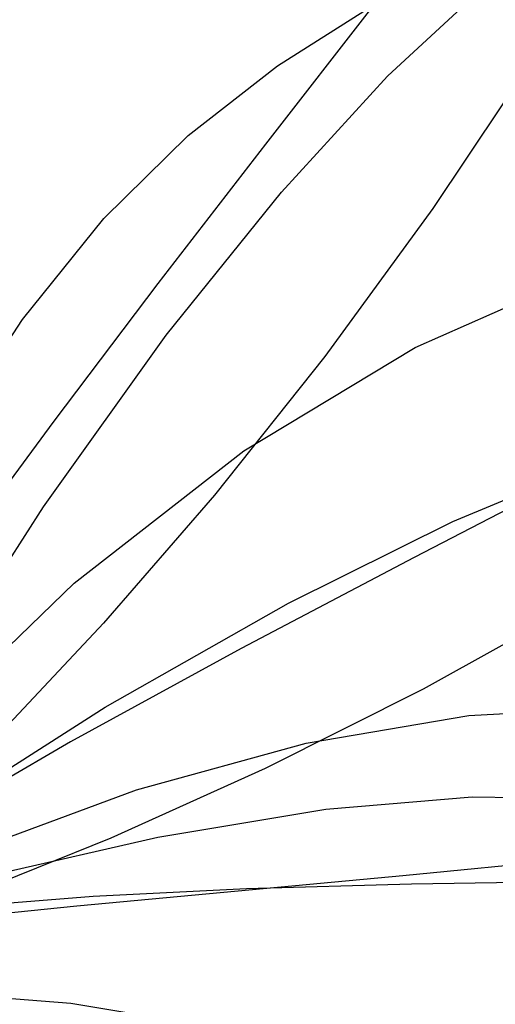
# Model space of a CAD drawing. Units: inches. Extents: x 3590 to 5167, y 65 to 1917.
# Tile 93 of 100: x 5053.48 to 5058.39, y 1778.86 to 1789.03. Entities that reach past the tile are written whole.
import ezdxf

# ---------------------------------------------------------------- set-up
doc = ezdxf.new("R2010")
doc.units = ezdxf.units.IN
for name, color, linetype, lineweight in [('A-ANNO-DIMS', 2, 'Continuous', 18), ('A-FLOR-PATT', 8, 'Continuous', 13), ('L-PLNT', 94, 'Continuous', 18)]:
    doc.layers.add(name, color=color, linetype=linetype, lineweight=lineweight)
doc.layers.add('DIENHOA', color=3, linetype='Continuous')
doc.styles.get("Standard").update_dxf_attribs({"font": 'arial.ttf'})
doc.dimstyles.new('ISO-25', dxfattribs={"dimtxt": 9, "dimasz": 2.5, "dimexe": 1.25, "dimexo": 0.625, "dimtad": 1, "dimdec": 1, "dimlunit": 3, "dimtxsty": 'Standard', "dimcen": 2.5, "dimadec": 0, "dimazin": 0, "dimtfac": 1, "dimtdec": 1, "dimtmove": 0, "dimatfit": 3, "dimfxl": 1, "dimarcsym": 0})

# ---------------------------------------------------------------- blocks, each defined once
blk = doc.blocks.new('Cay03_mb')
at = {"layer": 'DIENHOA'}
for p, q in [((290.63, 243.24), (363.38, 275.41)), ((218.51, 199.79), (290.63, 243.24)), ((146.96, 144.09), (218.51, 199.79)), ((363.69, 192.89), (290.19, 154.87)), ((290.19, 154.87), (217.38, 116.61)), ((75.94, 75.22), (146.96, 144.09)), ((217.38, 116.61), (145.48, 77.28)), ((145.48, 77.28), (74.74, 36.09)), ((252.97, 48.94), (314.63, 54.14)), ((314.63, 54.14), (369.18, 53.28)), ((182.2, 37.2), (252.97, 48.94)), ((100.34, 18.45), (182.2, 37.2)), ((289.03, 17.44), (219.62, 15.45)), ((361.61, 18.5), (289.03, 17.44)), ((219.62, 15.45), (154.97, 12.22)), ((154.97, 12.22), (96.66, 7.47))]:
    blk.add_line(p, q, dxfattribs=at)
for points in [[(384.28, 437.45), (342.25, 367.83), (298.14, 301.71), (252.56, 239.37), (206.11, 181.11), (159.39, 127.21), (113.01, 77.96), (67.57, 33.64), (23.69, -5.44)], [(23.69, -5.44), (79.88, 91.71), (134.12, 176.21), (185.81, 248.4), (234.31, 308.65), (279.02, 357.33), (319.33, 394.78), (354.62, 421.37), (384.28, 437.45)], [(273.24, 387.35), (227.6, 328.83), (182.25, 270.12), (138.39, 212.28), (97.23, 156.36), (59.96, 103.43), (27.8, 54.57), (1.94, 10.82), (-16.39, -26.73)], [(-16.39, -26.73), (21.41, 64.22), (57.05, 140.27), (91.37, 203.26), (125.24, 255.05), (159.51, 297.5), (195.03, 332.46), (232.65, 361.79), (273.24, 387.35)], [(496.74, 224.01), (429.38, 178.44), (361.6, 136.93), (294.07, 99.46), (227.46, 66.07), (162.44, 36.74), (99.68, 11.49), (39.84, -9.67), (-16.39, -26.73)], [(-16.39, -26.73), (75.38, 37.88), (160.06, 91.82), (237.27, 135.67), (306.57, 170.01), (367.58, 195.44), (419.88, 212.52), (463.07, 221.85), (496.74, 224.01)], [(23.69, -5.44), (99.27, 29.67), (173.22, 57.09), (244.79, 76.69), (313.26, 88.31), (377.88, 91.81), (437.93, 87.02), (492.67, 73.8), (541.37, 52)], [(541.37, 52), (484.11, 42.89), (421.18, 34.83), (354.36, 27.58), (285.41, 20.89), (216.1, 14.49), (148.2, 8.14), (83.47, 1.58), (23.69, -5.44)], [(-16.39, -26.73), (66.95, -26.58), (145.58, -32.71), (218.77, -44.94), (285.79, -63.12), (345.92, -87.06), (398.42, -116.6), (442.57, -151.57), (477.63, -191.79)]]:
    blk.add_lwpolyline(points, dxfattribs=at)
blk = doc.blocks.new('*D322')
at = {"layer": 'A-ANNO-DIMS', "color": 0, "lineweight": -2, "transparency": 16777216}
for p, q in [((5035.744, 1766.184), (5035.744, 1761.199)), ((5064.812, 1766.184), (5064.812, 1761.199)), ((5038.244, 1762.449), (5062.312, 1762.449)), ((5064.812, 1762.449), (5166.991, 1762.449))]:
    blk.add_line(p, q, dxfattribs=at)
at = {"layer": 'A-ANNO-DIMS', "color": 0, "transparency": 16777216}
for points in [[(5038.244, 1762.866), (5038.244, 1762.032), (5035.744, 1762.449)], [(5062.312, 1762.866), (5062.312, 1762.032), (5064.812, 1762.449)]]:
    blk.add_solid(points, dxfattribs=at)
at = {"layer": 'Defpoints', "color": 0, "transparency": 16777216}
for p in [(5035.744, 1766.809), (5064.812, 1766.809), (5064.812, 1762.449)]:
    blk.add_point(p, dxfattribs=at)
at = {"layer": 'A-ANNO-DIMS', "color": 0, "transparency": 16777216, "insert": (5117.152, 1767.669), "char_height": 9, "attachment_point": 5}
blk.add_mtext('PLANT 2\'-5" TYP.', dxfattribs=at)
blk = doc.blocks.new('*D323')
at = {"layer": 'A-ANNO-DIMS', "color": 0, "lineweight": -2, "transparency": 16777216}
for p, q in [((5069.172, 1795.216), (5069.172, 1874.95)), ((5065.437, 1795.216), (5070.422, 1795.216)), ((5069.172, 1769.309), (5069.172, 1792.716)), ((5065.437, 1766.809), (5070.422, 1766.809))]:
    blk.add_line(p, q, dxfattribs=at)
at = {"layer": 'A-ANNO-DIMS', "color": 0, "transparency": 16777216}
for points in [[(5068.756, 1792.716), (5069.589, 1792.716), (5069.172, 1795.216)], [(5068.756, 1769.309), (5069.589, 1769.309), (5069.172, 1766.809)]]:
    blk.add_solid(points, dxfattribs=at)
at = {"layer": 'Defpoints', "color": 0, "transparency": 16777216}
for p in [(5064.812, 1795.216), (5069.172, 1795.216), (5064.812, 1766.809)]:
    blk.add_point(p, dxfattribs=at)
at = {"layer": 'A-ANNO-DIMS', "color": 0, "transparency": 16777216, "insert": (5063.894, 1836.333), "char_height": 9, "attachment_point": 5, "rotation": 90}
blk.add_mtext('2\'-4 1/2" TYP.', dxfattribs=at)

msp = doc.modelspace()

# ---------------------------------------------------------------- hatches: boundary and pattern name
at = {"layer": 'A-FLOR-PATT', "transparency": 33554687}
h = msp.add_hatch(dxfattribs=at)
h.set_pattern_fill('AR-HBONE', color=256, scale=0.2)
h.set_pattern_definition([(45, (-588.972, 0), (0, 28.73682), [60.96, -20.32]), (135, (-574.604, 14.368), (3e-15, 28.73682), [60.96, -20.32])])
h.paths.add_polyline_path([(5071.274, 1796.999), (4933.274, 1796.999), (4933.274, 1753.999), (4962.774, 1753.999, -0.414214), (4928.774, 1719.999), (4933.274, 1718.999), (4933.274, 1334.999), (5071.274, 1334.999)])
h.paths.add_polyline_path([(4951.78, 1521.077), (4951.715, 1521.04), (4951.563, 1520.895)], flags=16)
h.paths.add_polyline_path([(4952.267, 1521.376), (4952.198, 1521.371), (4952.198, 1521.356)], flags=0)
h.paths.add_polyline_path([(4967.051, 1529.728), (4965.231, 1528.694), (4963.411, 1527.714), (4961.756, 1526.851), (4963.589, 1527.449), (4964.036, 1527.478), (4962.975, 1527.249), (4961.76, 1526.852), (4959.792, 1525.834), (4958.005, 1524.895), (4956.24, 1523.93), (4954.504, 1522.919), (4954.129, 1522.682), (4953.361, 1521.997), (4953.366, 1521.998), (4953.605, 1522.064), (4955.106, 1522.761), (4956.921, 1523.434), (4958.678, 1523.915), (4960.358, 1524.2), (4961.945, 1524.286), (4964.171, 1524.108), (4965.958, 1523.309), (4963.863, 1522.976), (4965.187, 1522.499), (4963.366, 1522.497), (4961.545, 1522.487), (4959.764, 1522.461), (4958.304, 1522.419), (4957.974, 1522.388), (4956.307, 1522.232), (4954.718, 1522.071), (4953.251, 1521.899), (4953.525, 1521.623), (4954.331, 1521.379), (4956.243, 1521.23), (4958.039, 1520.93), (4959.684, 1520.483), (4961.16, 1519.896), (4963.107, 1518.8), (4964.393, 1517.325), (4962.973, 1517.726), (4964.558, 1516.661), (4965.407, 1515.708), (4963.507, 1516.322), (4961.68, 1517.005), (4959.935, 1517.745), (4958.282, 1518.528), (4956.732, 1519.343), (4955.295, 1520.175), (4954.672, 1520.572), (4954.513, 1520.627), (4955.658, 1519.318), (4956.703, 1517.982), (4957.644, 1516.647), (4958.485, 1515.334), (4959.55, 1513.524), (4960.438, 1511.769), (4958.841, 1513.62), (4957.452, 1515.325), (4955.819, 1517.459), (4956.665, 1515.448), (4957.111, 1513.923), (4957.447, 1511.714), (4957.076, 1509.793), (4956.538, 1511.11), (4955.992, 1512.569), (4955.444, 1514.125), (4954.898, 1515.735), (4954.357, 1517.356), (4953.824, 1518.943), (4953.305, 1520.452), (4953.065, 1521.116), (4952.971, 1521.146), (4952.949, 1521.086), (4952.73, 1520.199), (4953.37, 1518.024), (4953.757, 1516.373), (4954.051, 1514.765), (4954.264, 1513.221), (4954.471, 1511.131), (4954.497, 1510.402), (4954.409, 1511.76), (4954.264, 1513.221), (4954.051, 1514.765), (4953.757, 1516.373), (4953.37, 1518.024), (4952.877, 1519.698), (4952.716, 1520.141), (4952.533, 1519.059), (4952.374, 1517.789), (4952.219, 1516.312), (4952.046, 1514.6), (4951.833, 1512.626), (4951.557, 1510.363), (4951.203, 1512.168), (4950.852, 1514.339), (4950.985, 1516.376), (4951.66, 1518.286), (4952.593, 1520.481), (4952.357, 1521.13), (4951.855, 1520.328), (4950.839, 1518.908), (4949.777, 1517.587), (4948.916, 1516.617), (4948.111, 1515.256), (4947.089, 1513.554), (4945.889, 1511.615), (4946.326, 1513.402), (4946.562, 1514.249), (4945.528, 1513.327), (4944.581, 1512.531), (4946.018, 1514.508), (4947.204, 1516.048), (4947.893, 1517.313), (4949.307, 1518.764), (4950.414, 1519.767), (4950.451, 1519.806), (4952.267, 1521.376), (4951.645, 1521.493), (4950.404, 1521.18), (4948.044, 1520.359), (4946.119, 1519.452), (4944.572, 1518.475), (4943.35, 1517.443), (4941.997, 1515.92), (4941.661, 1515.275), (4942.813, 1516.99), (4944.572, 1518.475), (4946.119, 1519.452), (4948.044, 1520.359), (4950.404, 1521.18), (4951.645, 1521.493), (4949.647, 1521.868), (4948.6, 1521.756), (4947.126, 1521.57), (4945.42, 1521.348), (4943.45, 1521.105), (4941.183, 1520.856), (4942.86, 1521.613), (4943.873, 1522.03), (4942.952, 1521.909), (4941.41, 1521.485), (4939.543, 1520.67), (4938.968, 1520.226), (4940.733, 1521.299), (4942.952, 1521.909), (4943.702, 1522.008), (4945.894, 1522.7), (4947.565, 1522.714), (4948.921, 1522.566), (4951.131, 1522.183), (4950.971, 1522.297), (4948.129, 1523.006), (4946.035, 1523.707), (4944.232, 1524.521), (4942.707, 1525.461), (4941.444, 1526.537), (4940.43, 1527.761), (4939.649, 1529.143), (4941.421, 1528.122), (4943.147, 1527.132), (4944.841, 1526.175), (4946.514, 1525.25), (4948.179, 1524.359), (4948.365, 1524.263), (4946.475, 1526.045), (4945.181, 1527.54), (4944.19, 1529.033), (4943.496, 1530.54), (4943.278, 1531.36), (4942.498, 1531.919), (4943.114, 1531.762), (4942.959, 1533.659), (4944.14, 1531.989), (4944.612, 1531.323), (4946.202, 1530.463), (4947.486, 1529.509), (4948.79, 1528.226), (4950.368, 1526.237), (4949.485, 1528.155), (4948.851, 1530.123), (4948.491, 1532.041), (4948.381, 1533.918), (4948.501, 1535.76), (4948.827, 1537.573), (4949.418, 1535.565), (4949.957, 1533.569), (4950.464, 1531.586), (4950.961, 1529.617), (4951.391, 1527.954), (4951.724, 1530.687), (4952.201, 1532.58), (4952.889, 1534.33), (4953.77, 1535.951), (4954.827, 1537.46), (4954.521, 1535.39), (4954.273, 1533.937), (4955.58, 1535.663), (4956.748, 1536.739), (4956.159, 1534.78), (4955.589, 1532.873), (4955.043, 1531.006), (4954.525, 1529.166), (4954.038, 1527.341), (4953.638, 1525.733), (4953.611, 1525.586), (4953.398, 1524.166), (4953.382, 1524.009), (4954.07, 1525.476), (4954.912, 1527.022), (4956.136, 1528.894), (4957.847, 1530.577), (4959.376, 1531.54), (4958.256, 1530.104), (4957.143, 1528.663), (4956.066, 1527.243), (4955.056, 1525.871), (4954.141, 1524.571), (4953.352, 1523.372), (4953.311, 1523.303), (4953.273, 1522.925), (4953.261, 1522.382), (4954.103, 1523.373), (4954.63, 1524.284), (4955.961, 1526.358), (4957.23, 1528.13), (4958.421, 1529.609), (4960.037, 1531.368), (4961.374, 1532.375), (4962.101, 1532.77), (4961.07, 1531.061), (4959.987, 1529.438), (4958.869, 1527.908), (4958.15, 1527.007), (4959.803, 1528.003), (4961.589, 1528.793), (4963.391, 1529.328), (4965.211, 1529.632)], flags=16)
h.paths.add_polyline_path([(4962.944, 1523.182), (4961.107, 1523.422), (4960.392, 1523.362), (4962.35, 1523.331)], flags=0)
h.paths.add_polyline_path([(5049.541, 1584.551), (5049.476, 1584.515), (5049.325, 1584.37)], flags=16)
h.paths.add_polyline_path([(5050.028, 1584.851), (5049.959, 1584.845), (5049.959, 1584.83)], flags=0)
h.paths.add_polyline_path([(5042.333, 1581.949), (5043.88, 1582.926), (5045.806, 1583.833), (5048.165, 1584.654), (5049.406, 1584.967), (5047.408, 1585.342), (5046.361, 1585.231), (5044.888, 1585.044), (5043.181, 1584.822), (5041.211, 1584.579), (5038.944, 1584.33), (5040.622, 1585.087), (5041.634, 1585.504), (5040.713, 1585.383), (5039.171, 1584.959), (5037.304, 1584.144), (5036.729, 1583.7), (5038.494, 1584.773), (5040.713, 1585.383), (5041.463, 1585.482), (5043.655, 1586.174), (5045.326, 1586.188), (5046.682, 1586.04), (5048.893, 1585.657), (5048.732, 1585.771), (5045.891, 1586.48), (5043.796, 1587.181), (5041.994, 1587.996), (5040.468, 1588.935), (5039.205, 1590.011), (5038.191, 1591.235), (5037.41, 1592.617), (5039.182, 1591.596), (5040.909, 1590.607), (5042.602, 1589.649), (5044.275, 1588.724), (5045.94, 1587.833), (5046.126, 1587.738), (5044.237, 1589.519), (5042.942, 1591.015), (5041.952, 1592.508), (5041.257, 1594.014), (5041.039, 1594.834), (5040.26, 1595.393), (5040.875, 1595.237), (5040.721, 1597.133), (5041.901, 1595.463), (5042.373, 1594.798), (5043.963, 1593.938), (5045.247, 1592.983), (5046.552, 1591.701), (5048.129, 1589.712), (5047.247, 1591.63), (5046.613, 1593.597), (5046.252, 1595.515), (5046.142, 1597.392), (5046.262, 1599.234), (5046.588, 1601.047), (5047.179, 1599.039), (5047.718, 1597.043), (5048.225, 1595.06), (5048.722, 1593.091), (5049.152, 1591.429), (5049.485, 1594.161), (5049.962, 1596.054), (5050.65, 1597.804), (5051.532, 1599.425), (5052.589, 1600.934), (5052.283, 1598.864), (5052.034, 1597.411), (5053.341, 1599.137), (5054.509, 1600.213), (5053.92, 1598.254), (5053.35, 1596.348), (5052.805, 1594.48), (5052.286, 1592.64), (5051.799, 1590.815), (5051.4, 1589.207), (5051.373, 1589.06), (5051.159, 1587.64), (5051.143, 1587.483), (5051.831, 1588.95), (5052.673, 1590.496), (5053.898, 1592.368), (5055.608, 1594.051), (5057.137, 1595.014), (5056.017, 1593.578), (5054.904, 1592.137), (5053.828, 1590.717), (5052.817, 1589.345), (5051.902, 1588.046), (5051.113, 1586.846), (5051.072, 1586.777), (5051.034, 1586.399), (5051.022, 1585.856), (5051.864, 1586.847), (5052.391, 1587.758), (5053.723, 1589.832), (5054.991, 1591.604), (5056.182, 1593.083), (5057.798, 1594.842), (5059.135, 1595.849), (5059.863, 1596.244), (5058.831, 1594.535), (5057.749, 1592.912), (5056.63, 1591.382), (5055.912, 1590.482), (5057.564, 1591.477), (5059.35, 1592.267), (5061.152, 1592.802), (5062.972, 1593.106), (5064.812, 1593.203), (5062.992, 1592.169), (5061.172, 1591.188), (5059.518, 1590.325), (5061.35, 1590.924), (5061.797, 1590.952), (5060.737, 1590.723), (5059.521, 1590.326), (5057.553, 1589.308), (5055.766, 1588.369), (5054.002, 1587.404), (5052.265, 1586.393), (5051.891, 1586.156), (5051.122, 1585.471), (5051.127, 1585.472), (5051.366, 1585.538), (5052.867, 1586.235), (5054.682, 1586.908), (5056.439, 1587.389), (5058.12, 1587.675), (5059.706, 1587.76), (5061.933, 1587.583), (5063.719, 1586.783), (5061.624, 1586.45), (5062.949, 1585.973), (5061.127, 1585.971), (5059.307, 1585.961), (5057.525, 1585.935), (5056.065, 1585.893), (5055.735, 1585.862), (5054.068, 1585.707), (5052.479, 1585.546), (5051.012, 1585.373), (5051.286, 1585.097), (5052.092, 1584.853), (5054.004, 1584.704), (5055.8, 1584.404), (5057.446, 1583.958), (5058.921, 1583.37), (5060.868, 1582.274), (5062.154, 1580.799), (5060.734, 1581.2), (5062.32, 1580.135), (5063.168, 1579.182), (5061.269, 1579.796), (5059.441, 1580.479), (5057.696, 1581.219), (5056.043, 1582.003), (5054.493, 1582.817), (5053.057, 1583.649), (5052.433, 1584.047), (5052.274, 1584.101), (5053.42, 1582.793), (5054.464, 1581.457), (5055.405, 1580.121), (5056.247, 1578.809), (5057.311, 1576.998), (5058.199, 1575.244), (5056.602, 1577.094), (5055.213, 1578.799), (5053.58, 1580.933), (5054.427, 1578.922), (5054.872, 1577.397), (5055.208, 1575.189), (5054.838, 1573.267), (5054.299, 1574.584), (5053.754, 1576.043), (5053.206, 1577.599), (5052.659, 1579.209), (5052.118, 1580.83), (5051.585, 1582.417), (5051.066, 1583.927), (5050.826, 1584.59), (5050.733, 1584.62), (5050.711, 1584.561), (5050.491, 1583.673), (5051.131, 1581.498), (5051.518, 1579.847), (5051.813, 1578.24), (5052.026, 1576.695), (5052.233, 1574.605), (5052.258, 1573.876), (5052.17, 1575.234), (5052.026, 1576.695), (5051.813, 1578.24), (5051.518, 1579.847), (5051.131, 1581.498), (5050.638, 1583.172), (5050.477, 1583.615), (5050.294, 1582.533), (5050.136, 1581.263), (5049.981, 1579.786), (5049.807, 1578.074), (5049.594, 1576.1), (5049.318, 1573.837), (5048.965, 1575.642), (5048.613, 1577.813), (5048.747, 1579.85), (5049.421, 1581.76), (5050.354, 1583.955), (5050.118, 1584.604), (5049.616, 1583.802), (5048.6, 1582.382), (5047.538, 1581.061), (5046.677, 1580.091), (5045.872, 1578.73), (5044.85, 1577.028), (5043.651, 1575.089), (5044.087, 1576.877), (5044.324, 1577.723), (5043.289, 1576.801), (5042.342, 1576.005), (5043.779, 1577.982), (5044.966, 1579.522), (5045.655, 1580.787), (5047.068, 1582.239), (5048.175, 1583.241), (5048.213, 1583.28), (5050.028, 1584.851), (5049.406, 1584.967), (5048.165, 1584.654), (5045.806, 1583.833), (5043.88, 1582.926), (5042.333, 1581.949), (5041.111, 1580.917), (5039.758, 1579.394), (5039.423, 1578.749), (5040.575, 1580.464)], flags=16)
h.paths.add_polyline_path([(4954.799, 1533.12), (4954.262, 1532.079), (4953.831, 1530.935), (4953.505, 1529.636), (4953.283, 1528.133), (4953.167, 1526.376), (4953.156, 1524.315), (4953.277, 1521.236), (4952.802, 1521.842), (4951.557, 1521.998), (4950.976, 1521.961), (4952.661, 1521.941), (4952.802, 1521.842), (4953.152, 1523.593), (4953.167, 1526.376), (4953.283, 1528.133), (4953.609, 1530.346), (4954.456, 1532.592)], flags=0)
h.paths.add_polyline_path([(5050.563, 1585.316), (5049.318, 1585.472), (5048.737, 1585.435), (5050.422, 1585.415), (5050.563, 1585.316), (5050.914, 1587.067), (5050.928, 1589.851), (5051.045, 1591.607), (5051.371, 1593.82), (5052.217, 1596.066), (5052.56, 1596.594), (5052.024, 1595.554), (5051.592, 1594.409), (5051.266, 1593.11), (5051.045, 1591.607), (5050.928, 1589.851), (5050.918, 1587.789), (5051.038, 1584.71)], flags=0)
h.paths.add_polyline_path([(5058.153, 1586.836), (5060.111, 1586.805), (5060.705, 1586.656), (5058.868, 1586.896)], flags=0)
h.paths.add_polyline_path([(5049.541, 1430.936), (5049.476, 1430.9), (5049.325, 1430.755)], flags=16)
h.paths.add_polyline_path([(5050.028, 1431.236), (5049.959, 1431.231), (5049.959, 1431.215)], flags=0)
h.paths.add_polyline_path([(5046.588, 1447.432), (5047.179, 1445.425), (5047.718, 1443.429), (5048.225, 1441.446), (5048.722, 1439.476), (5049.152, 1437.814), (5049.485, 1440.546), (5049.962, 1442.439), (5050.65, 1444.189), (5051.532, 1445.811), (5052.589, 1447.319), (5052.283, 1445.249), (5052.034, 1443.796), (5053.341, 1445.522), (5054.509, 1446.598), (5053.92, 1444.64), (5053.35, 1442.733), (5052.805, 1440.865), (5052.286, 1439.025), (5051.799, 1437.201), (5051.4, 1435.592), (5051.373, 1435.445), (5051.159, 1434.025), (5051.143, 1433.868), (5051.831, 1435.335), (5052.673, 1436.881), (5053.898, 1438.753), (5055.608, 1440.436), (5057.137, 1441.4), (5056.017, 1439.963), (5054.904, 1438.522), (5053.828, 1437.102), (5052.817, 1435.73), (5051.902, 1434.431), (5051.113, 1433.231), (5051.072, 1433.162), (5051.034, 1432.784), (5051.022, 1432.242), (5051.864, 1433.232), (5052.391, 1434.143), (5053.723, 1436.217), (5054.991, 1437.989), (5056.182, 1439.468), (5057.798, 1441.227), (5059.135, 1442.235), (5059.863, 1442.629), (5058.831, 1440.921), (5057.749, 1439.298), (5056.63, 1437.767), (5055.912, 1436.867), (5057.564, 1437.863), (5059.35, 1438.652), (5061.152, 1439.187), (5062.972, 1439.491), (5064.812, 1439.588), (5062.992, 1438.554), (5061.172, 1437.573), (5059.518, 1436.71), (5061.35, 1437.309), (5061.797, 1437.337), (5060.737, 1437.108), (5059.521, 1436.711), (5057.553, 1435.693), (5055.766, 1434.754), (5054.002, 1433.789), (5052.265, 1432.778), (5051.891, 1432.541), (5051.122, 1431.856), (5051.127, 1431.857), (5051.366, 1431.923), (5052.867, 1432.62), (5054.682, 1433.293), (5056.439, 1433.775), (5058.12, 1434.06), (5059.706, 1434.145), (5061.933, 1433.968), (5063.719, 1433.168), (5061.624, 1432.835), (5062.949, 1432.358), (5061.127, 1432.357), (5059.307, 1432.346), (5057.525, 1432.32), (5056.065, 1432.278), (5055.735, 1432.248), (5054.068, 1432.092), (5052.479, 1431.931), (5051.012, 1431.759), (5051.286, 1431.482), (5052.092, 1431.238), (5054.004, 1431.089), (5055.8, 1430.789), (5057.446, 1430.343), (5058.921, 1429.755), (5060.868, 1428.66), (5062.154, 1427.185), (5060.734, 1427.585), (5062.32, 1426.52), (5063.168, 1425.567), (5061.269, 1426.181), (5059.441, 1426.865), (5057.696, 1427.604), (5056.043, 1428.388), (5054.493, 1429.202), (5053.057, 1430.034), (5052.433, 1430.432), (5052.274, 1430.487), (5053.42, 1429.178), (5054.464, 1427.842), (5055.405, 1426.506), (5056.247, 1425.194), (5057.311, 1423.383), (5058.199, 1421.629), (5056.602, 1423.479), (5055.213, 1425.184), (5053.58, 1427.318), (5054.427, 1425.307), (5054.872, 1423.782), (5055.208, 1421.574), (5054.838, 1419.652), (5054.299, 1420.97), (5053.754, 1422.428), (5053.206, 1423.984), (5052.659, 1425.595), (5052.118, 1427.215), (5051.585, 1428.802), (5051.066, 1430.312), (5050.826, 1430.975), (5050.733, 1431.005), (5050.711, 1430.946), (5050.491, 1430.058), (5051.131, 1427.883), (5051.518, 1426.232), (5051.813, 1424.625), (5052.026, 1423.081), (5052.233, 1420.991), (5052.258, 1420.261), (5052.17, 1421.619), (5052.026, 1423.081), (5051.813, 1424.625), (5051.518, 1426.232), (5051.131, 1427.883), (5050.638, 1429.558), (5050.477, 1430.001), (5050.294, 1428.918), (5050.136, 1427.648), (5049.981, 1426.171), (5049.807, 1424.459), (5049.594, 1422.485), (5049.318, 1420.222), (5048.965, 1422.028), (5048.613, 1424.199), (5048.747, 1426.235), (5049.421, 1428.146), (5050.354, 1430.34), (5050.118, 1430.989), (5049.616, 1430.187), (5048.6, 1428.768), (5047.538, 1427.446), (5046.677, 1426.477), (5045.872, 1425.116), (5044.85, 1423.413), (5043.651, 1421.474), (5044.087, 1423.262), (5044.324, 1424.109), (5043.289, 1423.186), (5042.342, 1422.391), (5043.779, 1424.368), (5044.966, 1425.907), (5045.655, 1427.173), (5047.068, 1428.624), (5048.175, 1429.627), (5048.213, 1429.666), (5050.028, 1431.236), (5049.406, 1431.353), (5048.165, 1431.039), (5045.806, 1430.218), (5043.88, 1429.311), (5042.333, 1428.334), (5041.111, 1427.302), (5039.758, 1425.779), (5039.423, 1425.134), (5040.575, 1426.849), (5042.333, 1428.334), (5043.88, 1429.311), (5045.806, 1430.218), (5048.165, 1431.039), (5049.406, 1431.353), (5047.408, 1431.727), (5046.361, 1431.616), (5044.888, 1431.429), (5043.181, 1431.207), (5041.211, 1430.964), (5038.944, 1430.715), (5040.622, 1431.472), (5041.634, 1431.89), (5040.713, 1431.769), (5039.171, 1431.345), (5037.304, 1430.53), (5036.729, 1430.085), (5038.494, 1431.158), (5040.713, 1431.769), (5041.463, 1431.867), (5043.655, 1432.559), (5045.326, 1432.573), (5046.682, 1432.425), (5048.893, 1432.042), (5048.732, 1432.156), (5045.891, 1432.865), (5043.796, 1433.566), (5041.994, 1434.381), (5040.468, 1435.321), (5039.205, 1436.396), (5038.191, 1437.62), (5037.41, 1439.002), (5039.182, 1437.982), (5040.909, 1436.992), (5042.602, 1436.034), (5044.275, 1435.109), (5045.94, 1434.218), (5046.126, 1434.123), (5044.237, 1435.904), (5042.942, 1437.4), (5041.952, 1438.893), (5041.257, 1440.399), (5041.039, 1441.219), (5040.26, 1441.778), (5040.875, 1441.622), (5040.721, 1443.518), (5041.901, 1441.848), (5042.373, 1441.183), (5043.963, 1440.323), (5045.247, 1439.369), (5046.552, 1438.086), (5048.129, 1436.097), (5047.247, 1438.015), (5046.613, 1439.982), (5046.252, 1441.901), (5046.142, 1443.778), (5046.262, 1445.619)], flags=16)
h.paths.add_polyline_path([(5052.382, 1444.255), (5051.623, 1442.78), (5052.024, 1441.939), (5052.56, 1442.98)], flags=0)
h.paths.add_polyline_path([(5050.563, 1431.701), (5049.318, 1431.857), (5048.737, 1431.821), (5050.422, 1431.8)], flags=0)
h.paths.add_polyline_path([(5058.153, 1433.221), (5060.111, 1433.19), (5060.705, 1433.041), (5058.868, 1433.281)], flags=0)
h.paths.add_polyline_path([(5049.541, 1352.285), (5049.476, 1352.249), (5049.325, 1352.104)], flags=16)
h.paths.add_polyline_path([(5050.028, 1352.585), (5049.959, 1352.58), (5049.959, 1352.564)], flags=0)
h.paths.add_polyline_path([(5046.588, 1368.781), (5047.179, 1366.774), (5047.718, 1364.778), (5048.225, 1362.795), (5048.722, 1360.825), (5049.152, 1359.163), (5049.485, 1361.896), (5049.962, 1363.789), (5050.65, 1365.538), (5051.532, 1367.16), (5052.589, 1368.669), (5052.283, 1366.598), (5052.034, 1365.145), (5053.341, 1366.871), (5054.509, 1367.947), (5053.92, 1365.989), (5053.35, 1364.082), (5052.805, 1362.214), (5052.286, 1360.374), (5051.799, 1358.55), (5051.4, 1356.942), (5051.373, 1356.794), (5051.159, 1355.374), (5051.143, 1355.218), (5051.831, 1356.684), (5052.673, 1358.23), (5053.898, 1360.102), (5055.608, 1361.786), (5057.137, 1362.749), (5056.017, 1361.313), (5054.904, 1359.872), (5053.828, 1358.452), (5052.817, 1357.079), (5051.902, 1355.78), (5051.113, 1354.581), (5051.072, 1354.512), (5051.034, 1354.133), (5051.022, 1353.591), (5051.864, 1354.581), (5052.391, 1355.492), (5053.723, 1357.566), (5054.991, 1359.338), (5056.182, 1360.817), (5057.798, 1362.577), (5059.135, 1363.584), (5059.863, 1363.979), (5058.831, 1362.27), (5057.749, 1360.647), (5056.63, 1359.117), (5055.912, 1358.216), (5057.564, 1359.212), (5059.35, 1360.001), (5061.152, 1360.536), (5062.972, 1360.841), (5064.812, 1360.937), (5062.992, 1359.903), (5061.172, 1358.923), (5059.518, 1358.059), (5061.35, 1358.658), (5061.797, 1358.687), (5060.737, 1358.458), (5059.521, 1358.061), (5057.553, 1357.043), (5055.766, 1356.103), (5054.002, 1355.138), (5052.265, 1354.127), (5051.891, 1353.89), (5051.122, 1353.206), (5051.127, 1353.206), (5051.366, 1353.272), (5052.867, 1353.969), (5054.682, 1354.643), (5056.439, 1355.124), (5058.12, 1355.409), (5059.706, 1355.495), (5061.933, 1355.317), (5063.719, 1354.518), (5061.624, 1354.184), (5062.949, 1353.708), (5061.127, 1353.706), (5059.307, 1353.695), (5057.525, 1353.669), (5056.065, 1353.627), (5055.735, 1353.597), (5054.068, 1353.441), (5052.479, 1353.28), (5051.012, 1353.108), (5051.286, 1352.831), (5052.092, 1352.587), (5054.004, 1352.439), (5055.8, 1352.138), (5057.446, 1351.692), (5058.921, 1351.104), (5060.868, 1350.009), (5062.154, 1348.534), (5060.734, 1348.935), (5062.32, 1347.869), (5063.168, 1346.916), (5061.269, 1347.53), (5059.441, 1348.214), (5057.696, 1348.954), (5056.043, 1349.737), (5054.493, 1350.551), (5053.057, 1351.383), (5052.433, 1351.781), (5052.274, 1351.836), (5053.42, 1350.527), (5054.464, 1349.191), (5055.405, 1347.855), (5056.247, 1346.543), (5057.311, 1344.733), (5058.199, 1342.978), (5056.602, 1344.828), (5055.213, 1346.534), (5053.58, 1348.667), (5054.427, 1346.656), (5054.872, 1345.132), (5055.208, 1342.923), (5054.838, 1341.002), (5054.299, 1342.319), (5053.754, 1343.778), (5053.206, 1345.334), (5052.659, 1346.944), (5052.118, 1348.564), (5051.585, 1350.151), (5051.066, 1351.661), (5050.826, 1352.324), (5050.733, 1352.355), (5050.711, 1352.295), (5050.491, 1351.408), (5051.131, 1349.232), (5051.518, 1347.581), (5051.813, 1345.974), (5052.026, 1344.43), (5052.233, 1342.34), (5052.258, 1341.61), (5052.17, 1342.969), (5052.026, 1344.43), (5051.813, 1345.974), (5051.518, 1347.581), (5051.131, 1349.232), (5050.638, 1350.907), (5050.477, 1351.35), (5050.294, 1350.267), (5050.136, 1348.997), (5049.981, 1347.52), (5049.807, 1345.809), (5049.594, 1343.835), (5049.318, 1341.571), (5048.965, 1343.377), (5048.613, 1345.548), (5048.747, 1347.585), (5049.421, 1349.495), (5050.354, 1351.689), (5050.118, 1352.339), (5049.616, 1351.536), (5048.6, 1350.117), (5047.538, 1348.795), (5046.677, 1347.826), (5045.872, 1346.465), (5044.85, 1344.763), (5043.651, 1342.824), (5044.087, 1344.611), (5044.324, 1345.458), (5043.289, 1344.535), (5042.342, 1343.74), (5043.779, 1345.717), (5044.966, 1347.256), (5045.655, 1348.522), (5047.068, 1349.973), (5048.175, 1350.976), (5048.213, 1351.015), (5050.028, 1352.585), (5049.406, 1352.702), (5048.165, 1352.388), (5045.806, 1351.567), (5043.88, 1350.661), (5042.333, 1349.683), (5041.111, 1348.651), (5039.758, 1347.128), (5039.423, 1346.483), (5040.575, 1348.198), (5042.333, 1349.683), (5043.88, 1350.661), (5045.806, 1351.567), (5048.165, 1352.388), (5049.406, 1352.702), (5047.408, 1353.076), (5046.361, 1352.965), (5044.888, 1352.779), (5043.181, 1352.556), (5041.211, 1352.313), (5038.944, 1352.065), (5040.622, 1352.821), (5041.634, 1353.239), (5040.713, 1353.118), (5039.171, 1352.694), (5037.304, 1351.879), (5036.729, 1351.434), (5038.494, 1352.508), (5040.713, 1353.118), (5041.463, 1353.216), (5043.655, 1353.909), (5045.326, 1353.923), (5046.682, 1353.774), (5048.893, 1353.391), (5048.732, 1353.506), (5045.891, 1354.214), (5043.796, 1354.915), (5041.994, 1355.73), (5040.468, 1356.67), (5039.205, 1357.746), (5038.191, 1358.969), (5037.41, 1360.352), (5039.182, 1359.331), (5040.909, 1358.341), (5042.602, 1357.383), (5044.275, 1356.458), (5045.94, 1355.567), (5046.126, 1355.472), (5044.237, 1357.253), (5042.942, 1358.749), (5041.952, 1360.242), (5041.257, 1361.748), (5041.039, 1362.568), (5040.26, 1363.128), (5040.875, 1362.971), (5040.721, 1364.867), (5041.901, 1363.197), (5042.373, 1362.532), (5043.963, 1361.672), (5045.247, 1360.718), (5046.552, 1359.435), (5048.129, 1357.446), (5047.247, 1359.364), (5046.613, 1361.331), (5046.252, 1363.25), (5046.142, 1365.127), (5046.262, 1366.969)], flags=16)
h.paths.add_polyline_path([(5052.382, 1365.604), (5051.623, 1364.129), (5052.024, 1363.288), (5052.56, 1364.329)], flags=0)
h.paths.add_polyline_path([(4951.78, 1698.041), (4951.715, 1698.005), (4951.563, 1697.859)], flags=16)
h.paths.add_polyline_path([(4952.267, 1698.341), (4952.198, 1698.335), (4952.198, 1698.32)], flags=0)
h.paths.add_polyline_path([(4957.076, 1686.757), (4956.538, 1688.074), (4955.992, 1689.533), (4955.444, 1691.089), (4954.898, 1692.699), (4954.357, 1694.32), (4953.824, 1695.907), (4953.305, 1697.417), (4953.065, 1698.08), (4952.971, 1698.11), (4952.949, 1698.051), (4952.73, 1697.163), (4953.37, 1694.988), (4953.757, 1693.337), (4954.051, 1691.729), (4954.264, 1690.185), (4954.471, 1688.095), (4954.497, 1687.366), (4954.409, 1688.724), (4954.264, 1690.185), (4954.051, 1691.729), (4953.757, 1693.337), (4953.37, 1694.988), (4952.877, 1696.662), (4952.716, 1697.105), (4952.533, 1696.023), (4952.374, 1694.753), (4952.219, 1693.276), (4952.046, 1691.564), (4951.833, 1689.59), (4951.557, 1687.327), (4951.203, 1689.132), (4950.852, 1691.303), (4950.985, 1693.34), (4951.66, 1695.25), (4952.593, 1697.445), (4952.357, 1698.094), (4951.855, 1697.292), (4950.839, 1695.872), (4949.777, 1694.551), (4948.916, 1693.581), (4948.111, 1692.22), (4947.089, 1690.518), (4945.889, 1688.579), (4946.326, 1690.366), (4946.562, 1691.213), (4945.528, 1690.291), (4944.581, 1689.495), (4946.018, 1691.472), (4947.204, 1693.012), (4947.893, 1694.277), (4949.307, 1695.729), (4950.414, 1696.731), (4950.451, 1696.77), (4952.267, 1698.341), (4951.645, 1698.457), (4950.404, 1698.144), (4948.044, 1697.323), (4946.119, 1696.416), (4944.572, 1695.439), (4943.35, 1694.407), (4941.997, 1692.884), (4941.661, 1692.239), (4942.813, 1693.954), (4944.572, 1695.439), (4946.119, 1696.416), (4948.044, 1697.323), (4950.404, 1698.144), (4951.645, 1698.457), (4949.647, 1698.832), (4948.6, 1698.72), (4947.126, 1698.534), (4945.42, 1698.312), (4943.45, 1698.069), (4941.183, 1697.82), (4942.86, 1698.577), (4943.873, 1698.994), (4942.952, 1698.873), (4941.41, 1698.449), (4939.543, 1697.634), (4938.968, 1697.19), (4940.733, 1698.263), (4942.952, 1698.873), (4943.702, 1698.972), (4945.894, 1699.664), (4947.565, 1699.678), (4948.921, 1699.53), (4951.131, 1699.147), (4950.971, 1699.261), (4948.129, 1699.97), (4946.035, 1700.671), (4944.232, 1701.486), (4942.707, 1702.425), (4941.444, 1703.501), (4940.43, 1704.725), (4939.649, 1706.107), (4941.421, 1705.086), (4943.147, 1704.097), (4944.841, 1703.139), (4946.514, 1702.214), (4948.179, 1701.323), (4948.365, 1701.227), (4946.475, 1703.009), (4945.181, 1704.505), (4944.19, 1705.997), (4943.496, 1707.504), (4943.278, 1708.324), (4942.498, 1708.883), (4943.114, 1708.727), (4942.959, 1710.623), (4944.14, 1708.953), (4944.612, 1708.287), (4946.202, 1707.428), (4947.486, 1706.473), (4948.79, 1705.191), (4950.368, 1703.202), (4949.485, 1705.12), (4948.851, 1707.087), (4948.491, 1709.005), (4948.381, 1710.882), (4948.501, 1712.724), (4948.827, 1714.537), (4949.418, 1712.529), (4949.957, 1710.533), (4950.464, 1708.55), (4950.961, 1706.581), (4951.391, 1704.919), (4951.724, 1707.651), (4952.201, 1709.544), (4952.889, 1711.294), (4953.77, 1712.915), (4954.827, 1714.424), (4954.521, 1712.354), (4954.273, 1710.901), (4955.58, 1712.627), (4956.748, 1713.703), (4956.159, 1711.744), (4955.589, 1709.837), (4955.043, 1707.97), (4954.525, 1706.13), (4954.038, 1704.305), (4953.638, 1702.697), (4953.611, 1702.55), (4953.398, 1701.13), (4953.382, 1700.973), (4954.07, 1702.44), (4954.912, 1703.986), (4956.136, 1705.858), (4957.847, 1707.541), (4959.376, 1708.504), (4958.256, 1707.068), (4957.143, 1705.627), (4956.066, 1704.207), (4955.056, 1702.835), (4954.141, 1701.536), (4953.352, 1700.336), (4953.311, 1700.267), (4953.273, 1699.889), (4953.261, 1699.346), (4954.103, 1700.337), (4954.63, 1701.248), (4955.961, 1703.322), (4957.23, 1705.094), (4958.421, 1706.573), (4960.037, 1708.332), (4961.374, 1709.339), (4962.101, 1709.734), (4961.07, 1708.025), (4959.987, 1706.402), (4958.869, 1704.872), (4958.15, 1703.972), (4959.803, 1704.967), (4961.589, 1705.757), (4963.391, 1706.292), (4965.211, 1706.596), (4967.051, 1706.692), (4965.231, 1705.659), (4963.411, 1704.678), (4961.756, 1703.815), (4963.589, 1704.413), (4964.036, 1704.442), (4962.975, 1704.213), (4961.76, 1703.816), (4959.792, 1702.798), (4958.005, 1701.859), (4956.24, 1700.894), (4954.504, 1699.883), (4954.129, 1699.646), (4953.361, 1698.961), (4953.366, 1698.962), (4953.605, 1699.028), (4955.106, 1699.725), (4956.921, 1700.398), (4958.678, 1700.879), (4960.358, 1701.164), (4961.945, 1701.25), (4964.171, 1701.073), (4965.958, 1700.273), (4963.863, 1699.94), (4965.187, 1699.463), (4963.366, 1699.461), (4961.545, 1699.451), (4959.764, 1699.425), (4958.304, 1699.383), (4957.974, 1699.352), (4956.307, 1699.197), (4954.718, 1699.036), (4953.251, 1698.863), (4953.525, 1698.587), (4954.331, 1698.343), (4956.243, 1698.194), (4958.039, 1697.894), (4959.684, 1697.447), (4961.16, 1696.86), (4963.107, 1695.764), (4964.393, 1694.289), (4962.973, 1694.69), (4964.558, 1693.625), (4965.407, 1692.672), (4963.507, 1693.286), (4961.68, 1693.969), (4959.935, 1694.709), (4958.282, 1695.492), (4956.732, 1696.307), (4955.295, 1697.139), (4954.672, 1697.536), (4954.513, 1697.591), (4955.658, 1696.282), (4956.703, 1694.946), (4957.644, 1693.611), (4958.485, 1692.298), (4959.55, 1690.488), (4960.438, 1688.733), (4958.841, 1690.584), (4957.452, 1692.289), (4955.819, 1694.423), (4956.665, 1692.412), (4957.111, 1690.887), (4957.447, 1688.678)], flags=16)
h.paths.add_polyline_path([(5050.563, 1353.05), (5049.318, 1353.207), (5048.737, 1353.17), (5050.422, 1353.15)], flags=0)
h.paths.add_polyline_path([(4951.78, 1351.486), (4951.715, 1351.45), (4951.563, 1351.305)], flags=16)
h.paths.add_polyline_path([(4952.267, 1351.786), (4952.198, 1351.78), (4952.198, 1351.765)], flags=0)
h.paths.add_polyline_path([(4954.827, 1367.869), (4954.521, 1365.799), (4954.273, 1364.346), (4955.58, 1366.072), (4956.748, 1367.148), (4956.159, 1365.19), (4955.589, 1363.283), (4955.043, 1361.415), (4954.525, 1359.575), (4954.038, 1357.751), (4953.638, 1356.142), (4953.611, 1355.995), (4953.398, 1354.575), (4953.382, 1354.418), (4954.07, 1355.885), (4954.912, 1357.431), (4956.136, 1359.303), (4957.847, 1360.986), (4959.376, 1361.95), (4958.256, 1360.513), (4957.143, 1359.072), (4956.066, 1357.652), (4955.056, 1356.28), (4954.141, 1354.981), (4953.352, 1353.781), (4953.311, 1353.712), (4953.273, 1353.334), (4953.261, 1352.792), (4954.103, 1353.782), (4954.63, 1354.693), (4955.961, 1356.767), (4957.23, 1358.539), (4958.421, 1360.018), (4960.037, 1361.777), (4961.374, 1362.785), (4962.101, 1363.179), (4961.07, 1361.471), (4959.987, 1359.848), (4958.869, 1358.317), (4958.15, 1357.417), (4959.803, 1358.413), (4961.589, 1359.202), (4963.391, 1359.737), (4965.211, 1360.041), (4967.051, 1360.138), (4965.231, 1359.104), (4963.411, 1358.123), (4961.756, 1357.26), (4963.589, 1357.859), (4964.036, 1357.887), (4962.975, 1357.658), (4961.76, 1357.261), (4959.792, 1356.243), (4958.005, 1355.304), (4956.24, 1354.339), (4954.504, 1353.328), (4954.129, 1353.091), (4953.361, 1352.406), (4953.366, 1352.407), (4953.605, 1352.473), (4955.106, 1353.17), (4956.921, 1353.843), (4958.678, 1354.325), (4960.358, 1354.61), (4961.945, 1354.695), (4964.171, 1354.518), (4965.958, 1353.718), (4963.863, 1353.385), (4965.187, 1352.908), (4963.366, 1352.907), (4961.545, 1352.896), (4959.764, 1352.87), (4958.304, 1352.828), (4957.974, 1352.798), (4956.307, 1352.642), (4954.718, 1352.481), (4953.251, 1352.309), (4953.525, 1352.032), (4954.331, 1351.788), (4956.243, 1351.639), (4958.039, 1351.339), (4959.684, 1350.893), (4961.16, 1350.305), (4963.107, 1349.21), (4964.393, 1347.735), (4962.973, 1348.135), (4964.558, 1347.07), (4965.407, 1346.117), (4963.507, 1346.731), (4961.68, 1347.414), (4959.935, 1348.154), (4958.282, 1348.938), (4956.732, 1349.752), (4955.295, 1350.584), (4954.672, 1350.982), (4954.513, 1351.036), (4955.658, 1349.728), (4956.703, 1348.392), (4957.644, 1347.056), (4958.485, 1345.744), (4959.55, 1343.933), (4960.438, 1342.179), (4958.841, 1344.029), (4957.452, 1345.734), (4955.819, 1347.868), (4956.665, 1345.857), (4957.111, 1344.332), (4957.447, 1342.124), (4957.076, 1340.202), (4956.538, 1341.52), (4955.992, 1342.978), (4955.444, 1344.534), (4954.898, 1346.145), (4954.357, 1347.765), (4953.824, 1349.352), (4953.305, 1350.862), (4953.065, 1351.525), (4952.971, 1351.555), (4952.949, 1351.496), (4952.73, 1350.608), (4953.37, 1348.433), (4953.757, 1346.782), (4954.051, 1345.175), (4954.264, 1343.631), (4954.471, 1341.541), (4954.497, 1340.811), (4954.409, 1342.169), (4954.264, 1343.631), (4954.051, 1345.175), (4953.757, 1346.782), (4953.37, 1348.433), (4952.877, 1350.108), (4952.716, 1350.551), (4952.533, 1349.468), (4952.374, 1348.198), (4952.219, 1346.721), (4952.046, 1345.009), (4951.833, 1343.035), (4951.557, 1340.772), (4951.203, 1342.578), (4950.852, 1344.749), (4950.985, 1346.785), (4951.66, 1348.696), (4952.593, 1350.89), (4952.357, 1351.539), (4951.855, 1350.737), (4950.839, 1349.318), (4949.777, 1347.996), (4948.916, 1347.027), (4948.111, 1345.665), (4947.089, 1343.963), (4945.889, 1342.024), (4946.326, 1343.812), (4946.562, 1344.659), (4945.528, 1343.736), (4944.581, 1342.941), (4946.018, 1344.918), (4947.204, 1346.457), (4947.893, 1347.723), (4949.307, 1349.174), (4950.414, 1350.177), (4950.451, 1350.216), (4952.267, 1351.786), (4951.645, 1351.903), (4950.404, 1351.589), (4948.044, 1350.768), (4946.119, 1349.861), (4944.572, 1348.884), (4943.35, 1347.852), (4941.997, 1346.329), (4941.661, 1345.684), (4942.813, 1347.399), (4944.572, 1348.884), (4946.119, 1349.861), (4948.044, 1350.768), (4950.404, 1351.589), (4951.645, 1351.903), (4949.647, 1352.277), (4948.6, 1352.166), (4947.126, 1351.979), (4945.42, 1351.757), (4943.45, 1351.514), (4941.183, 1351.265), (4942.86, 1352.022), (4943.873, 1352.44), (4942.952, 1352.319), (4941.41, 1351.895), (4939.543, 1351.08), (4938.968, 1350.635), (4940.733, 1351.708), (4942.952, 1352.319), (4943.702, 1352.417), (4945.894, 1353.109), (4947.565, 1353.123), (4948.921, 1352.975), (4951.131, 1352.592), (4950.971, 1352.706), (4948.129, 1353.415), (4946.035, 1354.116), (4944.232, 1354.931), (4942.707, 1355.871), (4941.444, 1356.946), (4940.43, 1358.17), (4939.649, 1359.552), (4941.421, 1358.532), (4943.147, 1357.542), (4944.841, 1356.584), (4946.514, 1355.659), (4948.179, 1354.768), (4948.365, 1354.673), (4946.475, 1356.454), (4945.181, 1357.95), (4944.19, 1359.443), (4943.496, 1360.949), (4943.278, 1361.769), (4942.498, 1362.328), (4943.114, 1362.172), (4942.959, 1364.068), (4944.14, 1362.398), (4944.612, 1361.733), (4946.202, 1360.873), (4947.486, 1359.919), (4948.79, 1358.636), (4950.368, 1356.647), (4949.485, 1358.565), (4948.851, 1360.532), (4948.491, 1362.451), (4948.381, 1364.328), (4948.501, 1366.169), (4948.827, 1367.982), (4949.418, 1365.975), (4949.957, 1363.979), (4950.464, 1361.995), (4950.961, 1360.026), (4951.391, 1358.364), (4951.724, 1361.096), (4952.201, 1362.989), (4952.889, 1364.739), (4953.77, 1366.361)], flags=16)
h.paths.add_polyline_path([(4954.799, 1363.53), (4954.262, 1362.489), (4953.831, 1361.344), (4953.505, 1360.045), (4953.283, 1358.543), (4953.167, 1356.786), (4953.156, 1354.724), (4953.277, 1351.646), (4952.802, 1352.251), (4951.557, 1352.407), (4950.976, 1352.371), (4952.661, 1352.35), (4952.802, 1352.251), (4953.152, 1354.002), (4953.167, 1356.786), (4953.283, 1358.543), (4953.609, 1360.755), (4954.456, 1363.001)], flags=0)
h.paths.add_polyline_path([(4952.802, 1698.806), (4951.557, 1698.962), (4950.976, 1698.925), (4952.661, 1698.905), (4952.802, 1698.806), (4953.152, 1700.557), (4953.167, 1703.34), (4953.283, 1705.097), (4953.609, 1707.31), (4954.456, 1709.556), (4954.799, 1710.084), (4954.262, 1709.043), (4953.831, 1707.899), (4953.505, 1706.6), (4953.283, 1705.097), (4953.167, 1703.34), (4953.156, 1701.279), (4953.277, 1698.2)], flags=0)
h.paths.add_polyline_path([(4962.944, 1700.146), (4961.107, 1700.386), (4960.392, 1700.326), (4962.35, 1700.295)], flags=0)
h.paths.add_polyline_path([(5058.153, 1354.57), (5060.111, 1354.539), (5060.705, 1354.391), (5058.868, 1354.631)], flags=0)
h.paths.add_polyline_path([(4962.944, 1353.591), (4961.107, 1353.831), (4960.392, 1353.771), (4962.35, 1353.74)], flags=0)
h.paths.add_polyline_path([(5049.541, 1778.72), (5049.476, 1778.684), (5049.325, 1778.539)], flags=16)
h.paths.add_polyline_path([(5050.028, 1779.02), (5049.959, 1779.014), (5049.959, 1778.999)], flags=0)
h.paths.add_polyline_path([(5052.258, 1768.045), (5052.17, 1769.403), (5052.026, 1770.864), (5051.813, 1772.409), (5051.518, 1774.016), (5051.131, 1775.667), (5050.638, 1777.341), (5050.477, 1777.784), (5050.294, 1776.702), (5050.136, 1775.432), (5049.981, 1773.955), (5049.807, 1772.243), (5049.594, 1770.269), (5049.318, 1768.006), (5048.965, 1769.811), (5048.613, 1771.982), (5048.747, 1774.019), (5049.421, 1775.929), (5050.354, 1778.124), (5050.118, 1778.773), (5049.616, 1777.971), (5048.6, 1776.551), (5047.538, 1775.23), (5046.677, 1774.26), (5045.872, 1772.899), (5044.85, 1771.197), (5043.651, 1769.258), (5044.087, 1771.046), (5044.324, 1771.892), (5043.289, 1770.97), (5042.342, 1770.174), (5043.779, 1772.151), (5044.966, 1773.691), (5045.655, 1774.956), (5047.068, 1776.408), (5048.175, 1777.41), (5048.213, 1777.449), (5050.028, 1779.02), (5049.406, 1779.136), (5048.165, 1778.823), (5045.806, 1778.002), (5043.88, 1777.095), (5042.333, 1776.118), (5041.111, 1775.086), (5039.758, 1773.563), (5039.423, 1772.918), (5040.575, 1774.633), (5042.333, 1776.118), (5043.88, 1777.095), (5045.806, 1778.002), (5048.165, 1778.823), (5049.406, 1779.136), (5047.408, 1779.511), (5046.361, 1779.4), (5044.888, 1779.213), (5043.181, 1778.991), (5041.211, 1778.748), (5038.944, 1778.499), (5040.622, 1779.256), (5041.634, 1779.673), (5040.713, 1779.552), (5039.171, 1779.128), (5037.304, 1778.313), (5036.729, 1777.869), (5038.494, 1778.942), (5040.713, 1779.552), (5041.463, 1779.651), (5043.655, 1780.343), (5045.326, 1780.357), (5046.682, 1780.209), (5048.893, 1779.826), (5048.732, 1779.94), (5045.891, 1780.649), (5043.796, 1781.35), (5041.994, 1782.165), (5040.468, 1783.104), (5039.205, 1784.18), (5038.191, 1785.404), (5037.41, 1786.786), (5039.182, 1785.765), (5040.909, 1784.776), (5042.602, 1783.818), (5044.275, 1782.893), (5045.94, 1782.002), (5046.126, 1781.907), (5044.237, 1783.688), (5042.942, 1785.184), (5041.952, 1786.677), (5041.257, 1788.183), (5041.039, 1789.003), (5040.26, 1789.562), (5040.875, 1789.406), (5040.721, 1791.302), (5041.901, 1789.632), (5042.373, 1788.967), (5043.963, 1788.107), (5045.247, 1787.152), (5046.552, 1785.87), (5048.129, 1783.881), (5047.247, 1785.799), (5046.613, 1787.766), (5046.252, 1789.684), (5046.142, 1791.561), (5046.262, 1793.403), (5046.588, 1795.216), (5047.179, 1793.208), (5047.718, 1791.213), (5048.225, 1789.229), (5048.722, 1787.26), (5049.152, 1785.598), (5049.485, 1788.33), (5049.962, 1790.223), (5050.65, 1791.973), (5051.532, 1793.594), (5052.589, 1795.103), (5052.283, 1793.033), (5052.034, 1791.58), (5053.341, 1793.306), (5054.509, 1794.382), (5053.92, 1792.423), (5053.35, 1790.517), (5052.805, 1788.649), (5052.286, 1786.809), (5051.799, 1784.984), (5051.4, 1783.376), (5051.373, 1783.229), (5051.159, 1781.809), (5051.143, 1781.652), (5051.831, 1783.119), (5052.673, 1784.665), (5053.898, 1786.537), (5055.608, 1788.22), (5057.137, 1789.183), (5056.017, 1787.747), (5054.904, 1786.306), (5053.828, 1784.886), (5052.817, 1783.514), (5051.902, 1782.215), (5051.113, 1781.015), (5051.072, 1780.946), (5051.034, 1780.568), (5051.022, 1780.025), (5051.864, 1781.016), (5052.391, 1781.927), (5053.723, 1784.001), (5054.991, 1785.773), (5056.182, 1787.252), (5057.798, 1789.011), (5059.135, 1790.018), (5059.863, 1790.413), (5058.831, 1788.704), (5057.749, 1787.081), (5056.63, 1785.551), (5055.912, 1784.651), (5057.564, 1785.646), (5059.35, 1786.436), (5061.152, 1786.971), (5062.972, 1787.275), (5064.812, 1787.372), (5062.992, 1786.338), (5061.172, 1785.357), (5059.518, 1784.494), (5061.35, 1785.093), (5061.797, 1785.121), (5060.737, 1784.892), (5059.521, 1784.495), (5057.553, 1783.477), (5055.766, 1782.538), (5054.002, 1781.573), (5052.265, 1780.562), (5051.891, 1780.325), (5051.122, 1779.64), (5051.127, 1779.641), (5051.366, 1779.707), (5052.867, 1780.404), (5054.682, 1781.077), (5056.439, 1781.558), (5058.12, 1781.844), (5059.706, 1781.929), (5061.933, 1781.752), (5063.719, 1780.952), (5061.624, 1780.619), (5062.949, 1780.142), (5061.127, 1780.14), (5059.307, 1780.13), (5057.525, 1780.104), (5056.065, 1780.062), (5055.735, 1780.031), (5054.068, 1779.876), (5052.479, 1779.715), (5051.012, 1779.542), (5051.286, 1779.266), (5052.092, 1779.022), (5054.004, 1778.873), (5055.8, 1778.573), (5057.446, 1778.127), (5058.921, 1777.539), (5060.868, 1776.443), (5062.154, 1774.968), (5060.734, 1775.369), (5062.32, 1774.304), (5063.168, 1773.351), (5061.269, 1773.965), (5059.441, 1774.648), (5057.696, 1775.388), (5056.043, 1776.172), (5054.493, 1776.986), (5053.057, 1777.818), (5052.433, 1778.216), (5052.274, 1778.27), (5053.42, 1776.962), (5054.464, 1775.626), (5055.405, 1774.29), (5056.247, 1772.978), (5057.311, 1771.167), (5058.199, 1769.413), (5056.602, 1771.263), (5055.213, 1772.968), (5053.58, 1775.102), (5054.427, 1773.091), (5054.872, 1771.566), (5055.208, 1769.358), (5054.838, 1767.436), (5054.299, 1768.753), (5053.754, 1770.212), (5053.206, 1771.768), (5052.659, 1773.378), (5052.118, 1774.999), (5051.585, 1776.586), (5051.066, 1778.096), (5050.826, 1778.759), (5050.733, 1778.789), (5050.711, 1778.73), (5050.491, 1777.842), (5051.131, 1775.667), (5051.518, 1774.016), (5051.813, 1772.409), (5052.026, 1770.864), (5052.233, 1768.774)], flags=16)
h.paths.add_polyline_path([(5050.563, 1779.485), (5049.318, 1779.641), (5048.737, 1779.604), (5050.422, 1779.584), (5050.563, 1779.485), (5050.914, 1781.236), (5050.928, 1784.02), (5051.045, 1785.776), (5051.371, 1787.989), (5052.217, 1790.235), (5052.56, 1790.763), (5052.024, 1789.723), (5051.592, 1788.578), (5051.266, 1787.279), (5051.045, 1785.776), (5050.928, 1784.02), (5050.918, 1781.958), (5051.038, 1778.879)], flags=0)
h.paths.add_polyline_path([(5058.153, 1781.005), (5060.111, 1780.974), (5060.705, 1780.825), (5058.868, 1781.065)], flags=0)

# ---------------------------------------------------------------- block references
at = {"layer": 'L-PLNT', "xscale": 0.0245452446402784, "yscale": 0.0245452446402784, "zscale": 0.0245452446402784}
msp.add_blockref('Cay03_mb', (5050.431, 1779.676), dxfattribs=at)

# ---------------------------------------------------------------- dimensions: what is measured, and where the dimension line sits
at = {"layer": 'A-ANNO-DIMS'}
dim = msp.add_linear_dim(base=(5069.172, 1795.216), p1=(5064.812, 1766.809), p2=(5064.812, 1795.216), angle=90, text='<> TYP.', dimstyle='ISO-25', override={"dimdec": 1, "dimlfac": 1, "dimrnd": 0, "dimzin": 1, "dimdsep": 46, "dimlunit": 4, "dimfrac": 2}, dxfattribs=at)
dim.commit()
dim.dimension.update_dxf_attribs({"geometry": '*D323', "text_midpoint": (5063.894, 1836.333)})
dim = msp.add_linear_dim(base=(5064.812, 1762.449), p1=(5035.744, 1766.809), p2=(5064.812, 1766.809), text='PLANT <> TYP.', dimstyle='ISO-25', override={"dimdec": 1, "dimlfac": 1, "dimrnd": 0, "dimzin": 1, "dimdsep": 46, "dimlunit": 4, "dimfrac": 2}, dxfattribs=at)
dim.commit()
dim.dimension.update_dxf_attribs({"geometry": '*D322', "text_midpoint": (5117.152, 1767.669)})

doc.saveas('drawing.dxf')
